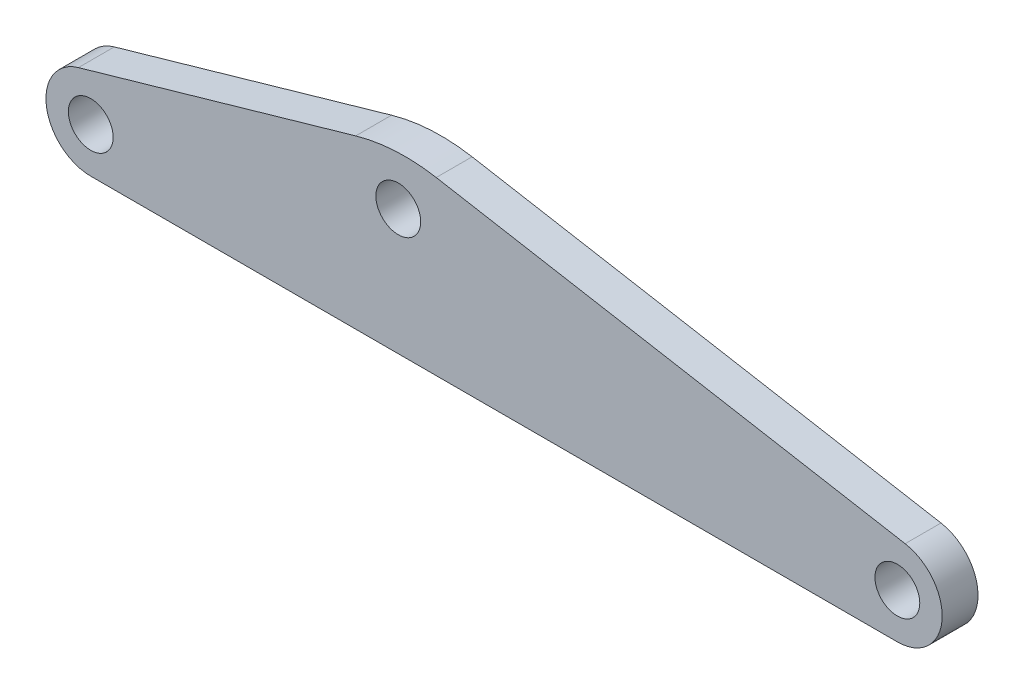
SolidWorks part; units mm, degrees
material "Plain Carbon Steel"
ref_plane "Front Plane" through (0, 0, 0) normal (0, 0, 1) x (1, 0, 0)
ref_plane "Top Plane" through (0, 0, 0) normal (0, 1, 0) x (1, 0, 0)
ref_plane "Right Plane" through (0, 0, 0) normal (1, 0, 0) x (0, 0, -1)
sketch "Link Profile Sketch" plane through (0, 0, 0) normal (0, 0, 1) x (1, 0, 0)
  line L0 (52.6018, 0) -> (-37.3982, 0)
  line L1 (-38.7764, 9.8063) -> (-7.8354, 18.6785)
  line L2 (1.1503, 19.1494) -> (53.47, 9.924)
  arc A0 (-38.7764, 9.8063) -> (-37.3982, 0) centre (-37.3982, 5) ccw
  arc A1 (52.6018, 0) -> (53.47, 9.924) centre (52.6018, 5) ccw
  circle A2 centre (-3.085, 14) radius 2.5
  circle A4 centre (-37.3982, 5) radius 2.5
  circle A5 centre (52.6018, 5) radius 2.5
  arc A6 (-7.8354, 18.6785) -> (1.1503, 19.1494) centre (-2.3227, -0.5467) cw
  dimension "D2" = 5
  dimension "D3" = 5
  dimension "D4" = 5
  dimension "D6" = 5
  dimension "D7" = 5
  dimension "D8" = 10
  dimension "D9" = 20
  dimension "D1" = 90
  dimension "14" = 14
  dimension "D5" = 16
  dimension "D10" = 37.3982
  dimension "D11" = 34.3132
extrude "Link Plate 4mm" add sketch "Link Profile Sketch" along normal blind 4
